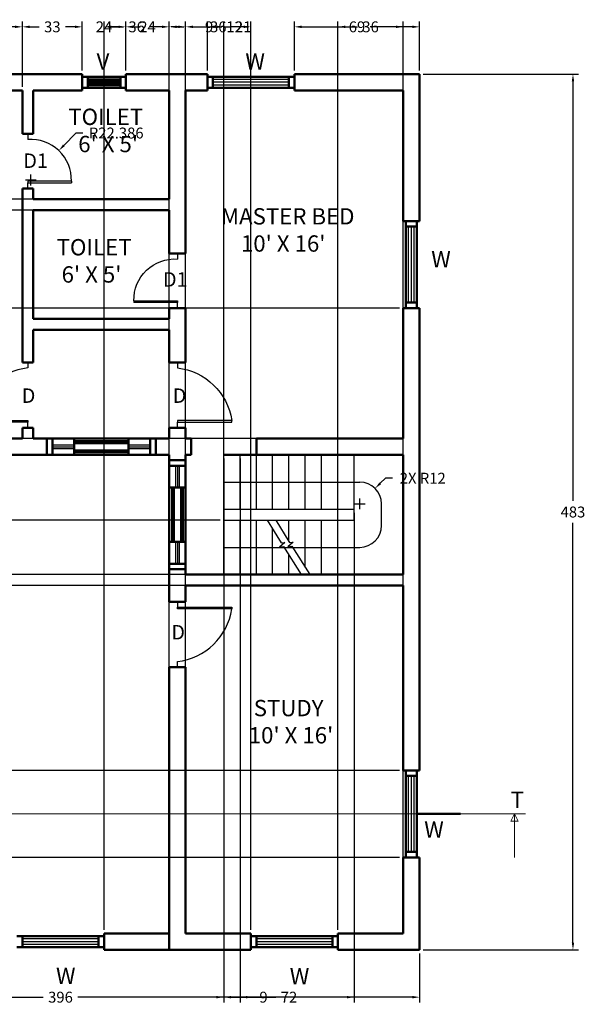
# Model space of a CAD drawing. Units: inches. Extents: x 853 to 2068, y 1026 to 2097.
# Tile 5 of 6: x 1756 to 2068, y 1026 to 1569. Entities that reach past the tile are written whole.
import ezdxf

# ---------------------------------------------------------------- set-up
doc = ezdxf.new("R2010")
doc.units = ezdxf.units.IN
doc.header["$MEASUREMENT"] = 0
for name, color, linetype, lineweight in [('A-ANNO-DIMS', 2, 'Continuous', 18), ('A-ANNO-SYMB', 2, 'Continuous', 18), ('A-ANNO-TEXT', 3, 'Continuous', 18), ('A-AREA-IDEN', 7, 'Continuous', 18), ('A-DOOR', 3, 'Continuous', 25), ('A-FLOR-STRS', 6, 'Continuous', 25), ('A-GLAZ', 4, 'Continuous', 25), ('A-WALL', 7, 'Continuous', 50)]:
    doc.layers.add(name, color=color, linetype=linetype, lineweight=lineweight)
doc.styles.get("Standard").update_dxf_attribs({"font": 'arial.ttf'})
doc.dimstyles.get("Standard").update_dxf_attribs({"dimtxt": 6, "dimasz": 4, "dimexe": 3, "dimexo": 2, "dimgap": 3, "dimtad": 0, "dimtih": 1, "dimtoh": 1, "dimdec": 0, "dimzin": 0, "dimdsep": 46, "dimlunit": 3, "dimtxsty": 'Standard', "dimcen": 3, "dimadec": 0, "dimazin": 0, "dimtfac": 1, "dimtdec": 0, "dimtofl": 0, "dimtmove": 0, "dimatfit": 3, "dimfxl": 1, "dimtolj": 1, "dimtzin": 0, "dimarcsym": 0})

# ---------------------------------------------------------------- blocks, each defined once
blk = doc.blocks.new('DOOR-D')
for p, q in [((0, 36), (0, 33)), ((0, 33), (30, 33)), ((0, 32), (0, 33)), ((30, 33), (30, 32)), ((30, 32), (0, 32)), ((0, 0), (0, 3))]:
    blk.add_line(p, q)
blk.add_arc((-4.1, 37.26), 34.5, 276.8214, 351.2366)
blk = doc.blocks.new('DOOR-D1')
for p, q in [((0, 30), (0, 27)), ((24, 4), (0, 4)), ((0, 4), (0, 3)), ((0, 0), (0, 3)), ((0, 3), (24, 3)), ((24, 4), (24, 3))]:
    blk.add_line(p, q)
blk.add_arc((1.62, 4.67), 22.39, 358.2784, 94.1594)
blk = doc.blocks.new('*D45')
at = {"layer": 'A-ANNO-DIMS', "color": 0, "lineweight": -2, "transparency": 16777216}
for p, q in [((1580.64, 1054.25), (1580.64, 1027.15)), ((1976.64, 1054.25), (1976.64, 1027.15)), ((1584.64, 1030.15), (1769.02, 1030.15)), ((1972.64, 1030.15), (1788.27, 1030.15))]:
    blk.add_line(p, q, dxfattribs=at)
at = {"layer": 'A-ANNO-DIMS', "color": 0, "transparency": 16777216}
for points in [[(1584.64, 1030.82), (1584.64, 1029.48), (1580.64, 1030.15)], [(1972.64, 1030.82), (1972.64, 1029.48), (1976.64, 1030.15)]]:
    blk.add_solid(points, dxfattribs=at)
at = {"layer": 'Defpoints', "color": 0, "transparency": 16777216}
for p in [(1580.64, 1056.25), (1976.64, 1056.25), (1976.64, 1030.15)]:
    blk.add_point(p, dxfattribs=at)
at = {"layer": 'A-ANNO-DIMS', "color": 0, "transparency": 16777216, "insert": (1778.64, 1030.15), "char_height": 6, "attachment_point": 5}
blk.add_mtext('\\A1;396', dxfattribs=at)
blk = doc.blocks.new('*D48')
at = {"layer": 'A-ANNO-DIMS', "color": 0, "lineweight": -2, "transparency": 16777216}
for p, q in [((1802.64, 1067.25), (1802.64, 1568.35)), ((1806.64, 1565.35), (1813.35, 1565.35)), ((1834.64, 1565.35), (1827.94, 1565.35)), ((1838.64, 1067.25), (1838.64, 1568.35))]:
    blk.add_line(p, q, dxfattribs=at)
at = {"layer": 'A-ANNO-DIMS', "color": 0, "transparency": 16777216}
for points in [[(1806.64, 1566.02), (1806.64, 1564.68), (1802.64, 1565.35)], [(1834.64, 1566.02), (1834.64, 1564.68), (1838.64, 1565.35)]]:
    blk.add_solid(points, dxfattribs=at)
at = {"layer": 'Defpoints', "color": 0, "transparency": 16777216}
for p in [(1838.64, 1565.35), (1802.64, 1065.25), (1838.64, 1065.25)]:
    blk.add_point(p, dxfattribs=at)
at = {"layer": 'A-ANNO-DIMS', "color": 0, "transparency": 16777216, "insert": (1820.64, 1565.35), "char_height": 6, "attachment_point": 5}
blk.add_mtext('\\A1;36', dxfattribs=at)
blk = doc.blocks.new('*D49')
at = {"layer": 'A-ANNO-DIMS', "color": 0, "lineweight": -2, "transparency": 16777216}
for p, q in [((1847.64, 1067.25), (1847.64, 1568.35)), ((1851.64, 1565.35), (1858.35, 1565.35)), ((1879.64, 1565.35), (1872.94, 1565.35)), ((1883.64, 1067.25), (1883.64, 1568.35))]:
    blk.add_line(p, q, dxfattribs=at)
at = {"layer": 'A-ANNO-DIMS', "color": 0, "transparency": 16777216}
for points in [[(1851.64, 1566.02), (1851.64, 1564.68), (1847.64, 1565.35)], [(1879.64, 1566.02), (1879.64, 1564.68), (1883.64, 1565.35)]]:
    blk.add_solid(points, dxfattribs=at)
at = {"layer": 'Defpoints', "color": 0, "transparency": 16777216}
for p in [(1883.64, 1565.35), (1847.64, 1065.25), (1883.64, 1065.25)]:
    blk.add_point(p, dxfattribs=at)
at = {"layer": 'A-ANNO-DIMS', "color": 0, "transparency": 16777216, "insert": (1865.64, 1565.35), "char_height": 6, "attachment_point": 5}
blk.add_mtext('\\A1;36', dxfattribs=at)
blk = doc.blocks.new('*D50')
at = {"layer": 'A-ANNO-DIMS', "color": 0, "lineweight": -2, "transparency": 16777216}
for p, q in [((1931.64, 1067.25), (1931.64, 1568.35)), ((1935.64, 1565.35), (1942.35, 1565.35)), ((1963.64, 1565.35), (1956.94, 1565.35)), ((1967.64, 1067.25), (1967.64, 1568.35))]:
    blk.add_line(p, q, dxfattribs=at)
at = {"layer": 'A-ANNO-DIMS', "color": 0, "transparency": 16777216}
for points in [[(1935.64, 1566.02), (1935.64, 1564.68), (1931.64, 1565.35)], [(1963.64, 1566.02), (1963.64, 1564.68), (1967.64, 1565.35)]]:
    blk.add_solid(points, dxfattribs=at)
at = {"layer": 'Defpoints', "color": 0, "transparency": 16777216}
for p in [(1967.64, 1565.35), (1931.64, 1065.25), (1967.64, 1065.25)]:
    blk.add_point(p, dxfattribs=at)
at = {"layer": 'A-ANNO-DIMS', "color": 0, "transparency": 16777216, "insert": (1949.64, 1565.35), "char_height": 6, "attachment_point": 5}
blk.add_mtext('\\A1;36', dxfattribs=at)
blk = doc.blocks.new('*D53')
at = {"layer": 'A-ANNO-DIMS', "color": 0, "lineweight": -2, "transparency": 16777216}
for p, q in [((1697.64, 1541.25), (1697.64, 1568.35)), ((1701.64, 1565.35), (1720.34, 1565.35)), ((1753.64, 1565.35), (1734.95, 1565.35)), ((1757.64, 1532.25), (1757.64, 1568.35))]:
    blk.add_line(p, q, dxfattribs=at)
at = {"layer": 'A-ANNO-DIMS', "color": 0, "transparency": 16777216}
for points in [[(1701.64, 1566.02), (1701.64, 1564.68), (1697.64, 1565.35)], [(1753.64, 1566.02), (1753.64, 1564.68), (1757.64, 1565.35)]]:
    blk.add_solid(points, dxfattribs=at)
at = {"layer": 'Defpoints', "color": 0, "transparency": 16777216}
for p in [(1757.64, 1565.35), (1697.64, 1539.25), (1757.64, 1530.25)]:
    blk.add_point(p, dxfattribs=at)
at = {"layer": 'A-ANNO-DIMS', "color": 0, "transparency": 16777216, "insert": (1727.64, 1565.35), "char_height": 6, "attachment_point": 5}
blk.add_mtext('\\A1;60', dxfattribs=at)
blk = doc.blocks.new('*D54')
at = {"layer": 'A-ANNO-DIMS', "color": 0, "lineweight": -2, "transparency": 16777216}
for p, q in [((1757.64, 1532.25), (1757.64, 1568.35)), ((1761.64, 1565.35), (1766.85, 1565.35)), ((1786.64, 1565.35), (1781.44, 1565.35)), ((1790.64, 1541.25), (1790.64, 1568.35))]:
    blk.add_line(p, q, dxfattribs=at)
at = {"layer": 'A-ANNO-DIMS', "color": 0, "transparency": 16777216}
for points in [[(1761.64, 1566.02), (1761.64, 1564.68), (1757.64, 1565.35)], [(1786.64, 1566.02), (1786.64, 1564.68), (1790.64, 1565.35)]]:
    blk.add_solid(points, dxfattribs=at)
at = {"layer": 'Defpoints', "color": 0, "transparency": 16777216}
for p in [(1790.64, 1565.35), (1790.64, 1539.25), (1757.64, 1530.25)]:
    blk.add_point(p, dxfattribs=at)
at = {"layer": 'A-ANNO-DIMS', "color": 0, "transparency": 16777216, "insert": (1774.14, 1565.35), "char_height": 6, "attachment_point": 5}
blk.add_mtext('\\A1;33', dxfattribs=at)
blk = doc.blocks.new('*D55')
at = {"layer": 'A-ANNO-DIMS', "color": 0, "lineweight": -2, "transparency": 16777216}
for p, q in [((1786.64, 1565.35), (1782.64, 1565.35)), ((1790.64, 1541.25), (1790.64, 1568.35)), ((1814.64, 1541.25), (1814.64, 1568.35)), ((1818.64, 1565.35), (1822.64, 1565.35))]:
    blk.add_line(p, q, dxfattribs=at)
at = {"layer": 'A-ANNO-DIMS', "color": 0, "transparency": 16777216}
for points in [[(1786.64, 1566.02), (1786.64, 1564.68), (1790.64, 1565.35)], [(1818.64, 1566.02), (1818.64, 1564.68), (1814.64, 1565.35)]]:
    blk.add_solid(points, dxfattribs=at)
at = {"layer": 'Defpoints', "color": 0, "transparency": 16777216}
for p in [(1814.64, 1565.35), (1790.64, 1539.25), (1814.64, 1539.25)]:
    blk.add_point(p, dxfattribs=at)
at = {"layer": 'A-ANNO-DIMS', "color": 0, "transparency": 16777216, "insert": (1802.64, 1565.35), "char_height": 6, "attachment_point": 5}
blk.add_mtext('\\A1;24', dxfattribs=at)
blk = doc.blocks.new('*D56')
at = {"layer": 'A-ANNO-DIMS', "color": 0, "lineweight": -2, "transparency": 16777216}
for p, q in [((1810.64, 1565.35), (1806.64, 1565.35)), ((1814.64, 1541.25), (1814.64, 1568.35)), ((1838.64, 1532.25), (1838.64, 1568.35)), ((1842.64, 1565.35), (1846.64, 1565.35))]:
    blk.add_line(p, q, dxfattribs=at)
at = {"layer": 'A-ANNO-DIMS', "color": 0, "transparency": 16777216}
for points in [[(1810.64, 1566.02), (1810.64, 1564.68), (1814.64, 1565.35)], [(1842.64, 1566.02), (1842.64, 1564.68), (1838.64, 1565.35)]]:
    blk.add_solid(points, dxfattribs=at)
at = {"layer": 'Defpoints', "color": 0, "transparency": 16777216}
for p in [(1838.64, 1565.35), (1814.64, 1539.25), (1838.64, 1530.25)]:
    blk.add_point(p, dxfattribs=at)
at = {"layer": 'A-ANNO-DIMS', "color": 0, "transparency": 16777216, "insert": (1826.64, 1565.35), "char_height": 6, "attachment_point": 5}
blk.add_mtext('\\A1;24', dxfattribs=at)
blk = doc.blocks.new('*D57')
at = {"layer": 'A-ANNO-DIMS', "color": 0, "lineweight": -2, "transparency": 16777216}
for p, q in [((1834.64, 1565.35), (1830.64, 1565.35)), ((1838.64, 1532.25), (1838.64, 1568.35)), ((1847.64, 1532.25), (1847.64, 1568.35)), ((1851.64, 1565.35), (1855.64, 1565.35))]:
    blk.add_line(p, q, dxfattribs=at)
at = {"layer": 'A-ANNO-DIMS', "color": 0, "transparency": 16777216}
for points in [[(1834.64, 1566.02), (1834.64, 1564.68), (1838.64, 1565.35)], [(1851.64, 1566.02), (1851.64, 1564.68), (1847.64, 1565.35)]]:
    blk.add_solid(points, dxfattribs=at)
at = {"layer": 'Defpoints', "color": 0, "transparency": 16777216}
for p in [(1847.64, 1565.35), (1838.64, 1530.25), (1847.64, 1530.25)]:
    blk.add_point(p, dxfattribs=at)
at = {"layer": 'A-ANNO-DIMS', "color": 0, "transparency": 16777216, "insert": (1860.61, 1565.35), "char_height": 6, "attachment_point": 5}
blk.add_mtext('\\A1;9', dxfattribs=at)
blk = doc.blocks.new('*D58')
at = {"layer": 'A-ANNO-DIMS', "color": 0, "lineweight": -2, "transparency": 16777216}
for p, q in [((1843.64, 1565.35), (1839.64, 1565.35)), ((1847.64, 1532.25), (1847.64, 1568.35)), ((1859.64, 1541.25), (1859.64, 1568.35)), ((1863.64, 1565.35), (1867.64, 1565.35))]:
    blk.add_line(p, q, dxfattribs=at)
at = {"layer": 'A-ANNO-DIMS', "color": 0, "transparency": 16777216}
for points in [[(1843.64, 1566.02), (1843.64, 1564.68), (1847.64, 1565.35)], [(1863.64, 1566.02), (1863.64, 1564.68), (1859.64, 1565.35)]]:
    blk.add_solid(points, dxfattribs=at)
at = {"layer": 'Defpoints', "color": 0, "transparency": 16777216}
for p in [(1859.64, 1565.35), (1859.64, 1539.25), (1847.64, 1530.25)]:
    blk.add_point(p, dxfattribs=at)
at = {"layer": 'A-ANNO-DIMS', "color": 0, "transparency": 16777216, "insert": (1874.63, 1565.35), "char_height": 6, "attachment_point": 5}
blk.add_mtext('\\A1;12', dxfattribs=at)
blk = doc.blocks.new('*D59')
at = {"layer": 'A-ANNO-DIMS', "color": 0, "lineweight": -2, "transparency": 16777216}
for p, q in [((1907.64, 1541.25), (1907.64, 1568.35)), ((1911.64, 1565.35), (1934.82, 1565.35)), ((1972.64, 1565.35), (1949.46, 1565.35)), ((1976.64, 1541.25), (1976.64, 1568.35))]:
    blk.add_line(p, q, dxfattribs=at)
at = {"layer": 'A-ANNO-DIMS', "color": 0, "transparency": 16777216}
for points in [[(1911.64, 1566.02), (1911.64, 1564.68), (1907.64, 1565.35)], [(1972.64, 1566.02), (1972.64, 1564.68), (1976.64, 1565.35)]]:
    blk.add_solid(points, dxfattribs=at)
at = {"layer": 'Defpoints', "color": 0, "transparency": 16777216}
for p in [(1976.64, 1565.35), (1907.64, 1539.25), (1976.64, 1539.25)]:
    blk.add_point(p, dxfattribs=at)
at = {"layer": 'A-ANNO-DIMS', "color": 0, "transparency": 16777216, "insert": (1942.14, 1565.35), "char_height": 6, "attachment_point": 5}
blk.add_mtext('\\A1;69', dxfattribs=at)
blk = doc.blocks.new('*D66')
at = {"layer": 'A-ANNO-DIMS', "color": 0, "lineweight": -2, "transparency": 16777216}
for p, q in [((1978.64, 1539.25), (2064.24, 1539.25)), ((2061.24, 1535.25), (2061.24, 1303.82)), ((2061.24, 1060.25), (2061.24, 1291.69)), ((1978.64, 1056.25), (2064.24, 1056.25))]:
    blk.add_line(p, q, dxfattribs=at)
at = {"layer": 'A-ANNO-DIMS', "color": 0, "transparency": 16777216}
for points in [[(2060.58, 1535.25), (2061.91, 1535.25), (2061.24, 1539.25)], [(2060.58, 1060.25), (2061.91, 1060.25), (2061.24, 1056.25)]]:
    blk.add_solid(points, dxfattribs=at)
at = {"layer": 'Defpoints', "color": 0, "transparency": 16777216}
for p in [(1976.64, 1539.25), (2061.24, 1539.25), (1976.64, 1056.25)]:
    blk.add_point(p, dxfattribs=at)
at = {"layer": 'A-ANNO-DIMS', "color": 0, "transparency": 16777216, "insert": (2061.24, 1297.75), "char_height": 6, "attachment_point": 5}
blk.add_mtext('\\A1;483', dxfattribs=at)
blk = doc.blocks.new('*D67')
at = {"layer": 'A-ANNO-DIMS', "color": 0, "lineweight": -2, "transparency": 16777216}
for p, q in [((1965.64, 1155.25), (1493.04, 1155.25)), ((1496.04, 1151.25), (1496.04, 1137.31)), ((1496.04, 1111.25), (1496.04, 1125.19)), ((1965.64, 1107.25), (1493.04, 1107.25))]:
    blk.add_line(p, q, dxfattribs=at)
at = {"layer": 'A-ANNO-DIMS', "color": 0, "transparency": 16777216}
for points in [[(1495.38, 1151.25), (1496.71, 1151.25), (1496.04, 1155.25)], [(1495.38, 1111.25), (1496.71, 1111.25), (1496.04, 1107.25)]]:
    blk.add_solid(points, dxfattribs=at)
at = {"layer": 'Defpoints', "color": 0, "transparency": 16777216}
for p in [(1496.04, 1155.25), (1967.64, 1155.25), (1967.64, 1107.25)]:
    blk.add_point(p, dxfattribs=at)
at = {"layer": 'A-ANNO-DIMS', "color": 0, "transparency": 16777216, "insert": (1496.04, 1131.25), "char_height": 6, "attachment_point": 5}
blk.add_mtext('\\A1;48', dxfattribs=at)
blk = doc.blocks.new('*D68')
at = {"layer": 'A-ANNO-DIMS', "color": 0, "lineweight": -2, "transparency": 16777216}
for p, q in [((1965.64, 1257.25), (1493.04, 1257.25)), ((1496.04, 1253.25), (1496.04, 1212.31)), ((1496.04, 1159.25), (1496.04, 1200.19)), ((1965.64, 1155.25), (1493.04, 1155.25))]:
    blk.add_line(p, q, dxfattribs=at)
at = {"layer": 'A-ANNO-DIMS', "color": 0, "transparency": 16777216}
for points in [[(1495.38, 1253.25), (1496.71, 1253.25), (1496.04, 1257.25)], [(1495.38, 1159.25), (1496.71, 1159.25), (1496.04, 1155.25)]]:
    blk.add_solid(points, dxfattribs=at)
at = {"layer": 'Defpoints', "color": 0, "transparency": 16777216}
for p in [(1496.04, 1257.25), (1967.64, 1257.25), (1967.64, 1155.25)]:
    blk.add_point(p, dxfattribs=at)
at = {"layer": 'A-ANNO-DIMS', "color": 0, "transparency": 16777216, "insert": (1496.04, 1206.25), "char_height": 6, "attachment_point": 5}
blk.add_mtext('\\A1;102', dxfattribs=at)
blk = doc.blocks.new('*D69')
at = {"layer": 'A-ANNO-DIMS', "color": 0, "lineweight": -2, "transparency": 16777216}
for p, q in [((1496.04, 1267.25), (1496.04, 1271.25)), ((1496.04, 1271.25), (1500.04, 1271.25)), ((1965.64, 1263.25), (1493.04, 1263.25)), ((1965.64, 1257.25), (1493.04, 1257.25)), ((1496.04, 1253.25), (1496.04, 1249.25))]:
    blk.add_line(p, q, dxfattribs=at)
at = {"layer": 'A-ANNO-DIMS', "color": 0, "transparency": 16777216}
for points in [[(1495.38, 1267.25), (1496.71, 1267.25), (1496.04, 1263.25)], [(1495.38, 1253.25), (1496.71, 1253.25), (1496.04, 1257.25)]]:
    blk.add_solid(points, dxfattribs=at)
at = {"layer": 'Defpoints', "color": 0, "transparency": 16777216}
for p in [(1496.04, 1263.25), (1967.64, 1263.25), (1967.64, 1257.25)]:
    blk.add_point(p, dxfattribs=at)
at = {"layer": 'A-ANNO-DIMS', "color": 0, "transparency": 16777216, "insert": (1505.02, 1271.25), "char_height": 6, "attachment_point": 5}
blk.add_mtext('\\A1;6', dxfattribs=at)
blk = doc.blocks.new('*D70')
at = {"layer": 'A-ANNO-DIMS', "color": 0, "lineweight": -2, "transparency": 16777216}
for p, q in [((1965.64, 1410.25), (1493.04, 1410.25)), ((1496.04, 1406.25), (1496.04, 1380.26)), ((1496.04, 1342.25), (1496.04, 1368.24)), ((1965.64, 1338.25), (1493.04, 1338.25))]:
    blk.add_line(p, q, dxfattribs=at)
at = {"layer": 'A-ANNO-DIMS', "color": 0, "transparency": 16777216}
for points in [[(1495.38, 1406.25), (1496.71, 1406.25), (1496.04, 1410.25)], [(1495.38, 1342.25), (1496.71, 1342.25), (1496.04, 1338.25)]]:
    blk.add_solid(points, dxfattribs=at)
at = {"layer": 'Defpoints', "color": 0, "transparency": 16777216}
for p in [(1496.04, 1410.25), (1967.64, 1410.25), (1967.64, 1338.25)]:
    blk.add_point(p, dxfattribs=at)
at = {"layer": 'A-ANNO-DIMS', "color": 0, "transparency": 16777216, "insert": (1496.04, 1374.25), "char_height": 6, "attachment_point": 5}
blk.add_mtext('\\A1;72', dxfattribs=at)
blk = doc.blocks.new('*D71')
at = {"layer": 'A-ANNO-DIMS', "color": 0, "lineweight": -2, "transparency": 16777216}
for p, q in [((1496.04, 1474.25), (1496.04, 1478.25)), ((1496.04, 1478.25), (1500.04, 1478.25)), ((1836.64, 1470.25), (1493.04, 1470.25)), ((1836.64, 1464.25), (1493.04, 1464.25)), ((1496.04, 1460.25), (1496.04, 1456.25))]:
    blk.add_line(p, q, dxfattribs=at)
at = {"layer": 'A-ANNO-DIMS', "color": 0, "transparency": 16777216}
for points in [[(1495.38, 1474.25), (1496.71, 1474.25), (1496.04, 1470.25)], [(1495.38, 1460.25), (1496.71, 1460.25), (1496.04, 1464.25)]]:
    blk.add_solid(points, dxfattribs=at)
at = {"layer": 'Defpoints', "color": 0, "transparency": 16777216}
for p in [(1496.04, 1470.25), (1838.64, 1470.25), (1838.64, 1464.25)]:
    blk.add_point(p, dxfattribs=at)
at = {"layer": 'A-ANNO-DIMS', "color": 0, "transparency": 16777216, "insert": (1505.02, 1478.25), "char_height": 6, "attachment_point": 5}
blk.add_mtext('\\A1;6', dxfattribs=at)
blk = doc.blocks.new('*D72')
at = {"layer": 'A-ANNO-DIMS', "color": 0, "lineweight": -2, "transparency": 16777216}
for p, q in [((1847.64, 1265.25), (1847.64, 1568.35)), ((1851.64, 1565.35), (1864.64, 1565.35)), ((1868.64, 1265.25), (1868.64, 1568.35)), ((1868.64, 1565.35), (1872.64, 1565.35))]:
    blk.add_line(p, q, dxfattribs=at)
at = {"layer": 'A-ANNO-DIMS', "color": 0, "transparency": 16777216}
for points in [[(1851.64, 1566.02), (1851.64, 1564.68), (1847.64, 1565.35)], [(1864.64, 1566.02), (1864.64, 1564.68), (1868.64, 1565.35)]]:
    blk.add_solid(points, dxfattribs=at)
at = {"layer": 'Defpoints', "color": 0, "transparency": 16777216}
for p in [(1868.64, 1565.35), (1847.64, 1263.25), (1868.64, 1263.25)]:
    blk.add_point(p, dxfattribs=at)
at = {"layer": 'A-ANNO-DIMS', "color": 0, "transparency": 16777216, "insert": (1879.41, 1565.35), "char_height": 6, "attachment_point": 5}
blk.add_mtext('\\A1;21', dxfattribs=at)
blk = doc.blocks.new('*D73')
at = {"layer": 'A-ANNO-DIMS', "color": 0, "lineweight": -2, "transparency": 16777216}
for p, q in [((1868.64, 1327.25), (1868.64, 1027.15)), ((1877.64, 1327.25), (1877.64, 1027.15)), ((1864.64, 1030.15), (1860.64, 1030.15)), ((1881.64, 1030.15), (1885.64, 1030.15))]:
    blk.add_line(p, q, dxfattribs=at)
at = {"layer": 'A-ANNO-DIMS', "color": 0, "transparency": 16777216}
for points in [[(1864.64, 1030.82), (1864.64, 1029.48), (1868.64, 1030.15)], [(1881.64, 1030.82), (1881.64, 1029.48), (1877.64, 1030.15)]]:
    blk.add_solid(points, dxfattribs=at)
at = {"layer": 'Defpoints', "color": 0, "transparency": 16777216}
for p in [(1868.64, 1329.25), (1877.64, 1329.25), (1877.64, 1030.15)]:
    blk.add_point(p, dxfattribs=at)
at = {"layer": 'A-ANNO-DIMS', "color": 0, "transparency": 16777216, "insert": (1890.61, 1030.15), "char_height": 6, "attachment_point": 5}
blk.add_mtext('\\A1;9', dxfattribs=at)
blk = doc.blocks.new('*D74')
at = {"layer": 'A-ANNO-DIMS', "color": 0, "lineweight": -2, "transparency": 16777216}
for p, q in [((1868.64, 1297.25), (1868.64, 1027.15)), ((1940.64, 1297.25), (1940.64, 1027.15)), ((1872.64, 1030.15), (1897.4, 1030.15)), ((1936.64, 1030.15), (1911.88, 1030.15))]:
    blk.add_line(p, q, dxfattribs=at)
at = {"layer": 'A-ANNO-DIMS', "color": 0, "transparency": 16777216}
for points in [[(1872.64, 1030.82), (1872.64, 1029.48), (1868.64, 1030.15)], [(1936.64, 1030.82), (1936.64, 1029.48), (1940.64, 1030.15)]]:
    blk.add_solid(points, dxfattribs=at)
at = {"layer": 'Defpoints', "color": 0, "transparency": 16777216}
for p in [(1868.64, 1299.25), (1940.64, 1299.25), (1940.64, 1030.15)]:
    blk.add_point(p, dxfattribs=at)
at = {"layer": 'A-ANNO-DIMS', "color": 0, "transparency": 16777216, "insert": (1904.64, 1030.15), "char_height": 6, "attachment_point": 5}
blk.add_mtext('\\A1;72', dxfattribs=at)
blk = doc.blocks.new('*D75')
at = {"layer": 'A-ANNO-DIMS', "color": 0, "lineweight": -2, "transparency": 16777216}
for p, q in [((1866.64, 1293.25), (1493.04, 1293.25)), ((1496.04, 1289.25), (1496.04, 1284.32)), ((1496.04, 1267.25), (1496.04, 1272.19)), ((1866.64, 1263.25), (1493.04, 1263.25))]:
    blk.add_line(p, q, dxfattribs=at)
at = {"layer": 'A-ANNO-DIMS', "color": 0, "transparency": 16777216}
for points in [[(1495.38, 1289.25), (1496.71, 1289.25), (1496.04, 1293.25)], [(1495.38, 1267.25), (1496.71, 1267.25), (1496.04, 1263.25)]]:
    blk.add_solid(points, dxfattribs=at)
at = {"layer": 'Defpoints', "color": 0, "transparency": 16777216}
for p in [(1496.04, 1293.25), (1868.64, 1293.25), (1868.64, 1263.25)]:
    blk.add_point(p, dxfattribs=at)
at = {"layer": 'A-ANNO-DIMS', "color": 0, "transparency": 16777216, "insert": (1496.04, 1278.25), "char_height": 6, "attachment_point": 5}
blk.add_mtext('\\A1;30', dxfattribs=at)
blk = doc.blocks.new('*D119')
at = {"layer": 'A-ANNO-DIMS', "color": 0, "lineweight": -2, "transparency": 16777216}
for p, q in [((1787.05, 1506.78), (1780.52, 1499.97)), ((1791.05, 1506.78), (1787.05, 1506.78)), ((1762.27, 1477.92), (1762.27, 1483.92)), ((1759.27, 1480.92), (1765.27, 1480.92))]:
    blk.add_line(p, q, dxfattribs=at)
at = {"layer": 'A-ANNO-DIMS', "color": 0, "transparency": 16777216}
blk.add_solid([(1780.04, 1500.44), (1781, 1499.51), (1777.75, 1497.09)], dxfattribs=at)
at = {"layer": 'Defpoints', "color": 0, "transparency": 16777216}
for p in [(1777.75, 1497.09), (1762.27, 1480.92)]:
    blk.add_point(p, dxfattribs=at)
at = {"layer": 'A-ANNO-DIMS', "color": 0, "transparency": 16777216, "insert": (1809.37, 1506.78), "char_height": 6, "attachment_point": 5}
blk.add_mtext('\\A1;R22.386', dxfattribs=at)
blk = doc.blocks.new('*D120')
at = {"layer": 'A-ANNO-DIMS', "color": 0, "lineweight": -2, "transparency": 16777216}
for p, q in [((1957.78, 1316.39), (1954.96, 1313.57)), ((1961.78, 1316.39), (1957.78, 1316.39)), ((1943.64, 1299.25), (1943.64, 1305.25)), ((1940.64, 1302.25), (1946.64, 1302.25))]:
    blk.add_line(p, q, dxfattribs=at)
at = {"layer": 'A-ANNO-DIMS', "color": 0, "transparency": 16777216}
blk.add_solid([(1954.48, 1314.04), (1955.43, 1313.09), (1952.13, 1310.74)], dxfattribs=at)
at = {"layer": 'Defpoints', "color": 0, "transparency": 16777216}
for p in [(1952.13, 1310.74), (1943.64, 1302.25)]:
    blk.add_point(p, dxfattribs=at)
at = {"layer": 'A-ANNO-DIMS', "color": 0, "transparency": 16777216, "insert": (1978.42, 1316.39), "char_height": 6, "attachment_point": 5}
blk.add_mtext('\\A1;2X R12', dxfattribs=at)

msp = doc.modelspace()

# ---------------------------------------------------------------- linework, layer by layer
at = {"layer": 'A-ANNO-SYMB'}
for p, q in [((1522.142, 1131.2513), (2035.142, 1131.2513)), ((2027.0037, 1127.2513), (2029.0037, 1131.2513)), ((2029.0037, 1131.2513), (2029.0037, 1107.2513)), ((2029.0037, 1131.2513), (2029.0037, 1127.2513)), ((2031.0037, 1127.2513), (2029.0037, 1131.2513)), ((2029.0037, 1131.2513), (2029.0037, 1127.2513)), ((2029.0037, 1127.2513), (2027.0037, 1127.2513)), ((2029.0037, 1127.2513), (2031.0037, 1127.2513))]:
    msp.add_line(p, q, dxfattribs=at)
at = {"layer": 'A-FLOR-STRS'}
for p, q in [((1868.642, 1299.2513), (1868.642, 1329.2513)), ((1877.642, 1299.2513), (1877.642, 1329.2513)), ((1886.642, 1299.2513), (1886.642, 1329.2513)), ((1895.642, 1299.2513), (1895.642, 1329.2513)), ((1904.642, 1299.2513), (1904.642, 1329.2513)), ((1913.642, 1299.2513), (1913.642, 1329.2513)), ((1922.642, 1299.2513), (1922.642, 1329.2513)), ((1931.642, 1299.2513), (1931.642, 1329.2513)), ((1940.642, 1293.2513), (1940.642, 1329.2513)), ((1868.642, 1314.2513), (1943.642, 1314.2513)), ((1868.642, 1299.2513), (1940.642, 1299.2513)), ((1955.642, 1290.2513), (1955.642, 1302.2513)), ((1868.642, 1263.2513), (1868.642, 1293.2513)), ((1868.642, 1293.2513), (1940.642, 1293.2513)), ((1877.642, 1263.2513), (1877.642, 1293.2513)), ((1886.642, 1263.2513), (1886.642, 1293.2513)), ((1892.592, 1293.2513), (1900.4102, 1280.7803)), ((1897.3131, 1293.2513), (1904.642, 1281.5607)), ((1904.642, 1281.5607), (1904.642, 1293.2513)), ((1913.642, 1267.2046), (1913.642, 1293.2513)), ((1922.642, 1263.2513), (1922.642, 1293.2513)), ((1931.642, 1263.2513), (1931.642, 1293.2513)), ((1895.642, 1263.2513), (1895.642, 1288.3861)), ((1895.642, 1288.3861), (1900.4102, 1280.7803)), ((1868.642, 1278.2513), (1943.642, 1278.2513)), ((1902.4034, 1280.9455), (1899.3864, 1278.3191)), ((1899.3864, 1278.3191), (1901.7016, 1278.7204)), ((1900.4102, 1280.7803), (1902.4034, 1280.9455)), ((1901.7016, 1278.7204), (1911.3994, 1263.2513)), ((1907.0048, 1281.1363), (1903.9878, 1278.5099)), ((1903.9878, 1278.5099), (1906.303, 1278.9112)), ((1904.642, 1281.5607), (1905.0116, 1280.9712)), ((1905.0116, 1280.9712), (1907.0048, 1281.1363)), ((1906.303, 1278.9112), (1916.1204, 1263.2513)), ((1904.642, 1263.2513), (1904.642, 1274.03))]:
    msp.add_line(p, q, dxfattribs=at)
for centre, start, end in [((1943.642, 1302.2513), 0, 90), ((1943.642, 1290.2513), 270, 0)]:
    msp.add_arc(centre, 12, start, end, dxfattribs=at)
at = {"layer": 'A-GLAZ'}
for p, q in [((1811.642, 1535.7513), (1793.642, 1535.7513)), ((1811.642, 1535.2513), (1793.642, 1535.2513)), ((1811.642, 1534.2513), (1793.642, 1534.2513)), ((1811.642, 1533.7513), (1793.642, 1533.7513)), ((1904.642, 1536.2513), (1862.642, 1536.2513)), ((1904.642, 1534.7513), (1862.642, 1534.7513)), ((1904.642, 1533.2513), (1862.642, 1533.2513)), ((1970.642, 1413.2513), (1970.642, 1455.2513)), ((1972.142, 1413.2513), (1972.142, 1455.2513)), ((1973.642, 1413.2513), (1973.642, 1455.2513)), ((1774.142, 1334.7513), (1786.142, 1334.7513)), ((1774.142, 1333.7513), (1786.142, 1333.7513)), ((1774.142, 1332.7513), (1786.142, 1332.7513)), ((1816.142, 1334.7513), (1828.142, 1334.7513)), ((1816.142, 1333.7513), (1828.142, 1333.7513)), ((1816.142, 1332.7513), (1828.142, 1332.7513)), ((1842.142, 1323.2513), (1842.142, 1311.2513)), ((1843.142, 1323.2513), (1843.142, 1311.2513)), ((1844.142, 1323.2513), (1844.142, 1311.2513)), ((1842.142, 1281.2513), (1842.142, 1269.2513)), ((1843.142, 1281.2513), (1843.142, 1269.2513)), ((1844.142, 1281.2513), (1844.142, 1269.2513)), ((1970.642, 1110.2513), (1970.642, 1152.2513)), ((1972.142, 1110.2513), (1972.142, 1152.2513)), ((1973.642, 1110.2513), (1973.642, 1152.2513)), ((1799.642, 1062.2513), (1757.642, 1062.2513)), ((1799.642, 1060.7513), (1757.642, 1060.7513)), ((1799.642, 1059.2513), (1757.642, 1059.2513)), ((1928.642, 1062.2513), (1886.642, 1062.2513)), ((1928.642, 1060.7513), (1886.642, 1060.7513)), ((1928.642, 1059.2513), (1886.642, 1059.2513))]:
    msp.add_line(p, q, dxfattribs=at)
at = {"layer": 'A-WALL'}
for p, q in [((1697.642, 1539.2513), (1790.642, 1539.2513)), ((1790.642, 1539.2513), (1790.642, 1530.2513)), ((1802.642, 1537.7513), (1790.642, 1537.7513)), ((1793.642, 1537.7513), (1793.642, 1531.7513)), ((1814.642, 1537.7513), (1802.642, 1537.7513)), ((1811.642, 1537.7513), (1811.642, 1531.7513)), ((1814.642, 1539.2513), (1859.642, 1539.2513)), ((1814.642, 1539.2513), (1814.642, 1530.2513)), ((1859.642, 1539.2513), (1859.642, 1530.2513)), ((1907.642, 1537.7513), (1859.642, 1537.7513)), ((1862.642, 1537.7513), (1862.642, 1531.7513)), ((1904.642, 1537.7513), (1904.642, 1531.7513)), ((1907.642, 1539.2513), (1976.642, 1539.2513)), ((1907.642, 1539.2513), (1907.642, 1530.2513)), ((1976.642, 1458.2513), (1976.642, 1539.2513)), ((1802.642, 1531.7513), (1790.642, 1531.7513)), ((1802.642, 1536.2513), (1793.642, 1536.2513)), ((1802.642, 1534.7513), (1793.642, 1534.7513)), ((1802.642, 1533.2513), (1793.642, 1533.2513)), ((1811.642, 1536.2513), (1802.642, 1536.2513)), ((1811.642, 1534.7513), (1802.642, 1534.7513)), ((1811.642, 1533.2513), (1802.642, 1533.2513)), ((1814.642, 1531.7513), (1802.642, 1531.7513)), ((1907.642, 1531.7513), (1859.642, 1531.7513)), ((1697.642, 1530.2513), (1757.642, 1530.2513)), ((1697.642, 1530.2513), (1757.642, 1530.2513)), ((1757.642, 1530.2513), (1757.642, 1506.2513)), ((1763.642, 1530.2513), (1790.642, 1530.2513)), ((1763.642, 1530.2513), (1763.642, 1506.2513)), ((1790.642, 1530.2513), (1766.642, 1530.2513)), ((1814.642, 1530.2513), (1838.642, 1530.2513)), ((1838.642, 1530.2513), (1814.642, 1530.2513)), ((1838.642, 1470.2513), (1838.642, 1530.2513)), ((1847.642, 1530.2513), (1859.642, 1530.2513)), ((1859.642, 1530.2513), (1847.642, 1530.2513)), ((1847.642, 1530.2513), (1847.642, 1440.2513)), ((1907.642, 1530.2513), (1967.642, 1530.2513)), ((1967.642, 1530.2513), (1907.642, 1530.2513)), ((1967.642, 1458.2513), (1967.642, 1530.2513)), ((1967.642, 1458.2513), (1967.642, 1530.2513)), ((1763.642, 1506.2513), (1757.642, 1506.2513)), ((1757.642, 1476.2513), (1757.642, 1380.2513)), ((1763.642, 1476.2513), (1757.642, 1476.2513)), ((1763.642, 1476.2513), (1763.642, 1470.2513)), ((1763.642, 1470.2513), (1838.642, 1470.2513)), ((1763.642, 1464.2513), (1763.642, 1404.2513)), ((1763.642, 1464.2513), (1838.642, 1464.2513)), ((1838.642, 1464.2513), (1838.642, 1440.2513)), ((1976.642, 1458.2513), (1967.642, 1458.2513)), ((1969.142, 1410.2513), (1969.142, 1458.2513)), ((1975.142, 1410.2513), (1975.142, 1458.2513)), ((1975.142, 1455.2513), (1969.142, 1455.2513)), ((1838.642, 1440.2513), (1847.642, 1440.2513)), ((1975.142, 1413.2513), (1969.142, 1413.2513)), ((1838.642, 1410.2513), (1838.642, 1404.2513)), ((1838.642, 1410.2513), (1847.642, 1410.2513)), ((1847.642, 1410.2513), (1847.642, 1380.2513)), ((1967.642, 1338.2513), (1967.642, 1410.2513)), ((1967.642, 1338.2513), (1967.642, 1410.2513)), ((1976.642, 1410.2513), (1967.642, 1410.2513)), ((1976.642, 1155.2513), (1976.642, 1410.2513)), ((1838.642, 1404.2513), (1763.642, 1404.2513)), ((1763.642, 1398.2513), (1763.642, 1380.2513)), ((1838.642, 1398.2513), (1763.642, 1398.2513)), ((1838.642, 1380.2513), (1838.642, 1398.2513)), ((1757.642, 1380.2513), (1763.642, 1380.2513)), ((1838.642, 1380.2513), (1847.642, 1380.2513)), ((1757.642, 1344.2513), (1763.642, 1344.2513)), ((1757.642, 1344.2513), (1757.642, 1338.2513)), ((1763.642, 1344.2513), (1763.642, 1338.2513)), ((1838.642, 1338.2513), (1838.642, 1344.2513)), ((1838.642, 1344.2513), (1847.642, 1344.2513)), ((1847.642, 1344.2513), (1847.642, 1338.2513)), ((1757.642, 1338.2513), (1634.642, 1338.2513)), ((1763.642, 1338.2513), (1769.642, 1338.2513)), ((1763.642, 1338.2513), (1769.642, 1338.2513)), ((1769.642, 1338.2513), (1838.642, 1338.2513)), ((1771.142, 1338.2513), (1771.142, 1329.2513)), ((1771.142, 1329.2513), (1771.142, 1338.2513)), ((1774.142, 1329.2513), (1774.142, 1338.2513)), ((1786.142, 1329.2513), (1786.142, 1338.2513)), ((1786.142, 1336.7513), (1816.142, 1336.7513)), ((1816.142, 1338.2513), (1816.142, 1329.2513)), ((1828.142, 1338.2513), (1828.142, 1329.2513)), ((1831.142, 1338.2513), (1831.142, 1329.2513)), ((1847.642, 1338.2513), (1850.642, 1338.2513)), ((1850.642, 1338.2513), (1850.642, 1329.2513)), ((1886.642, 1338.2513), (1967.642, 1338.2513)), ((1886.642, 1338.2513), (1886.642, 1329.2513)), ((1786.142, 1335.7513), (1816.142, 1335.7513)), ((1786.142, 1331.7513), (1816.142, 1331.7513)), ((1786.142, 1330.7513), (1816.142, 1330.7513)), ((1769.642, 1329.2513), (1634.642, 1329.2513)), ((1838.642, 1329.2513), (1769.642, 1329.2513)), ((1838.642, 1248.2513), (1838.642, 1329.2513)), ((1838.642, 1326.2513), (1847.642, 1326.2513)), ((1847.642, 1329.2513), (1850.642, 1329.2513)), ((1847.642, 1329.2513), (1847.642, 1263.2513)), ((1868.642, 1329.2513), (1967.642, 1329.2513)), ((1967.642, 1263.2513), (1967.642, 1329.2513)), ((1838.642, 1323.2513), (1847.642, 1323.2513)), ((1838.642, 1311.2513), (1847.642, 1311.2513)), ((1840.142, 1311.2513), (1840.142, 1281.2513)), ((1841.142, 1311.2513), (1841.142, 1281.2513)), ((1845.142, 1311.2513), (1845.142, 1281.2513)), ((1846.142, 1311.2513), (1846.142, 1281.2513)), ((1847.642, 1281.2513), (1838.642, 1281.2513)), ((1847.642, 1269.2513), (1838.642, 1269.2513)), ((1847.642, 1266.2513), (1838.642, 1266.2513)), ((1847.642, 1263.2513), (1967.642, 1263.2513)), ((1847.642, 1248.2513), (1847.642, 1257.2513)), ((1847.642, 1257.2513), (1967.642, 1257.2513)), ((1967.642, 1155.2513), (1967.642, 1257.2513)), ((1967.642, 1257.2513), (1967.642, 1155.2513)), ((1847.642, 1248.2513), (1838.642, 1248.2513)), ((1838.642, 1065.2513), (1838.642, 1212.2513)), ((1847.642, 1212.2513), (1838.642, 1212.2513)), ((1847.642, 1065.2513), (1847.642, 1212.2513)), ((1976.642, 1155.2513), (1967.642, 1155.2513)), ((1969.142, 1107.2513), (1969.142, 1155.2513)), ((1975.142, 1152.2513), (1969.142, 1152.2513)), ((1975.142, 1107.2513), (1975.142, 1155.2513)), ((1975.142, 1131.2513), (1999.142, 1131.2513)), ((1975.142, 1110.2513), (1969.142, 1110.2513)), ((1967.642, 1065.2513), (1967.642, 1107.2513)), ((1967.642, 1107.2513), (1967.642, 1065.2513)), ((1976.642, 1107.2513), (1967.642, 1107.2513)), ((1976.642, 1056.2513), (1976.642, 1107.2513)), ((1802.642, 1065.2513), (1838.642, 1065.2513)), ((1802.642, 1065.2513), (1802.642, 1056.2513)), ((1802.642, 1065.2513), (1802.642, 1056.2513)), ((1838.642, 1065.2513), (1838.642, 1056.2513)), ((1883.642, 1065.2513), (1847.642, 1065.2513)), ((1883.642, 1065.2513), (1883.642, 1056.2513)), ((1967.642, 1065.2513), (1931.642, 1065.2513)), ((1931.642, 1065.2513), (1931.642, 1056.2513)), ((1802.642, 1063.7513), (1754.642, 1063.7513)), ((1757.642, 1063.7513), (1757.642, 1057.7513)), ((1799.642, 1063.7513), (1799.642, 1057.7513)), ((1931.642, 1063.7513), (1883.642, 1063.7513)), ((1886.642, 1063.7513), (1886.642, 1057.7513)), ((1928.642, 1063.7513), (1928.642, 1057.7513)), ((1802.642, 1057.7513), (1754.642, 1057.7513)), ((1802.642, 1056.2513), (1883.642, 1056.2513)), ((1931.642, 1057.7513), (1883.642, 1057.7513)), ((1931.642, 1056.2513), (1976.642, 1056.2513))]:
    msp.add_line(p, q, dxfattribs=at)

# ---------------------------------------------------------------- block references
at = {"layer": 'A-DOOR'}
for name, p in [('DOOR-D1', (1760.642, 1476.251)), ('DOOR-D', (1843.142, 1212.251))]:
    msp.add_blockref(name, p, dxfattribs=at)
at = {"layer": 'A-DOOR', "extrusion": (0, 0, -1), "zscale": -1}
msp.add_blockref('DOOR-D1', (-1843.142, 1410.251), dxfattribs=at)
at = {"layer": 'A-DOOR', "rotation": 180}
msp.add_blockref('DOOR-D', (1760.642, 1380.2515), dxfattribs=at)
at = {"layer": 'A-DOOR', "extrusion": (0, 0, -1), "zscale": -1, "rotation": 180}
msp.add_blockref('DOOR-D', (-1843.142, 1380.2515), dxfattribs=at)

# ---------------------------------------------------------------- texts
at = {"layer": 'A-ANNO-TEXT', "attachment_point": 1}
for s, insert, char_height in [('V', (1798.5377, 1550.7406), 9), ('W', (1880.5941, 1550.7406), 9), ('D1', (1758.1488, 1495.5014), 8), ('W', (1983.0893, 1441.6756), 9), ('D1', (1835.1751, 1430.0269), 8), ('D', (1757.2785, 1365.9329), 8), ('D', (1840.5118, 1365.9329), 8), ('D', (1839.7871, 1235.434), 8), ('{\\fArial|b1|i0|c0|p34;T}', (2026.8981, 1143.5184), 9), ('W', (1979.2188, 1127.1152), 9), ('W', (1776.1521, 1046.4713), 9), ('W', (1905.075, 1046.1485), 9)]:
    msp.add_mtext_dynamic_manual_height_columns(s, width=85.037544, gutter_width=1, heights=[0], dxfattribs=dict(at, insert=insert, char_height=char_height))
at = {"layer": 'A-AREA-IDEN', "char_height": 9, "attachment_point": 1}
for s, insert in [("TOILET\\P  6' X 5'", (1782.9114, 1520.2153)), ("MASTER BED\\P    10' X 16'", (1867.143, 1465.3249)), (" TOILET\\P  6' X 5'", (1773.7545, 1448.281)), ("      STUDY\\P     10' X 16'", (1868.6985, 1194.1022))]:
    msp.add_mtext_dynamic_manual_height_columns(s, width=85.037544, gutter_width=1, heights=[0], dxfattribs=dict(at, insert=insert))

# ---------------------------------------------------------------- dimensions: what is measured, and where the dimension line sits
at = {"layer": 'A-ANNO-DIMS'}
for base, p1, p2, picture, middle in [((1757.642, 1565.3513), (1697.642, 1539.2513), (1757.642, 1530.2513), '*D53', (1727.642, 1565.3513)), ((1790.642, 1565.3513), (1757.642, 1530.2513), (1790.642, 1539.2513), '*D54', (1774.142, 1565.3513)), ((1814.642, 1565.3513), (1790.642, 1539.2513), (1814.642, 1539.2513), '*D55', (1802.642, 1565.3513)), ((1838.642, 1565.3513), (1802.642, 1065.2513), (1838.642, 1065.2513), '*D48', (1820.642, 1565.3513)), ((1838.642, 1565.3513), (1814.642, 1539.2513), (1838.642, 1530.2513), '*D56', (1826.642, 1565.3513)), ((1847.642, 1565.3513), (1838.642, 1530.2513), (1847.642, 1530.2513), '*D57', (1860.6148, 1565.3513)), ((1859.642, 1565.3513), (1847.642, 1530.2513), (1859.642, 1539.2513), '*D58', (1874.6264, 1565.3513)), ((1883.642, 1565.3513), (1847.642, 1065.2513), (1883.642, 1065.2513), '*D49', (1865.642, 1565.3513)), ((1868.642, 1565.3513), (1847.642, 1263.2513), (1868.642, 1263.2513), '*D72', (1879.4115, 1565.3513)), ((1976.642, 1565.3513), (1907.642, 1539.2513), (1976.642, 1539.2513), '*D59', (1942.142, 1565.3513)), ((1967.642, 1565.3513), (1931.642, 1065.2513), (1967.642, 1065.2513), '*D50', (1949.642, 1565.3513)), ((1877.642, 1030.1513), (1868.642, 1329.2513), (1877.642, 1329.2513), '*D73', (1890.6148, 1030.1513)), ((1940.642, 1030.1513), (1868.642, 1299.2513), (1940.642, 1299.2513), '*D74', (1904.642, 1030.1513)), ((1976.642, 1030.1513), (1580.642, 1056.2513), (1976.642, 1056.2513), '*D45', (1778.642, 1030.1513))]:
    dim = msp.add_linear_dim(base=base, p1=p1, p2=p2, dimstyle='Standard', override={"dimdec": 0, "dimlfac": 1, "dimrnd": 0, "dimzin": 0, "dimdsep": 46, "dimlunit": 2}, dxfattribs=at)
    dim.commit()
    dim.dimension.update_dxf_attribs({"geometry": picture, "text_midpoint": middle})
for base, p1, p2, picture, middle in [((2061.242, 1539.2513), (1976.642, 1056.2513), (1976.642, 1539.2513), '*D66', (2061.242, 1297.7513)), ((1496.042, 1470.2513), (1838.642, 1464.2513), (1838.642, 1470.2513), '*D71', (1505.0229, 1478.2513)), ((1496.042, 1410.2513), (1967.642, 1338.2513), (1967.642, 1410.2513), '*D70', (1496.042, 1374.2513)), ((1496.042, 1293.2513), (1868.642, 1263.2513), (1868.642, 1293.2513), '*D75', (1496.042, 1278.2513)), ((1496.042, 1263.2513), (1967.642, 1257.2513), (1967.642, 1263.2513), '*D69', (1505.0229, 1271.2513)), ((1496.042, 1257.2513), (1967.642, 1155.2513), (1967.642, 1257.2513), '*D68', (1496.042, 1206.2513)), ((1496.042, 1155.2513), (1967.642, 1107.2513), (1967.642, 1155.2513), '*D67', (1496.042, 1131.2513))]:
    dim = msp.add_linear_dim(base=base, p1=p1, p2=p2, angle=90, dimstyle='Standard', override={"dimdec": 0, "dimlfac": 1, "dimrnd": 0, "dimzin": 0, "dimdsep": 46, "dimlunit": 2}, dxfattribs=at)
    dim.commit()
    dim.dimension.update_dxf_attribs({"geometry": picture, "text_midpoint": middle})
dim = msp.add_radius_dim(center=(1762.2657, 1480.9238), mpoint=(1777.7548, 1497.0868), dimstyle='Standard', override={"dimdec": 3, "dimlfac": 1, "dimrnd": 0, "dimzin": 0, "dimdsep": 46, "dimlunit": 2}, dxfattribs=at)
dim.commit()
dim.dimension.update_dxf_attribs({"geometry": '*D119', "text_midpoint": (1809.3715, 1506.7845), "dimtype": 164})
dim = msp.add_radius_dim(center=(1943.642, 1302.2513), mpoint=(1952.1269, 1310.7369), text='2X <>', dimstyle='Standard', override={"dimdec": 0, "dimlfac": 1, "dimrnd": 0, "dimzin": 0, "dimdsep": 46, "dimlunit": 2}, dxfattribs=at)
dim.commit()
dim.dimension.update_dxf_attribs({"geometry": '*D120', "text_midpoint": (1978.4186, 1316.394)})

doc.saveas('drawing.dxf')
